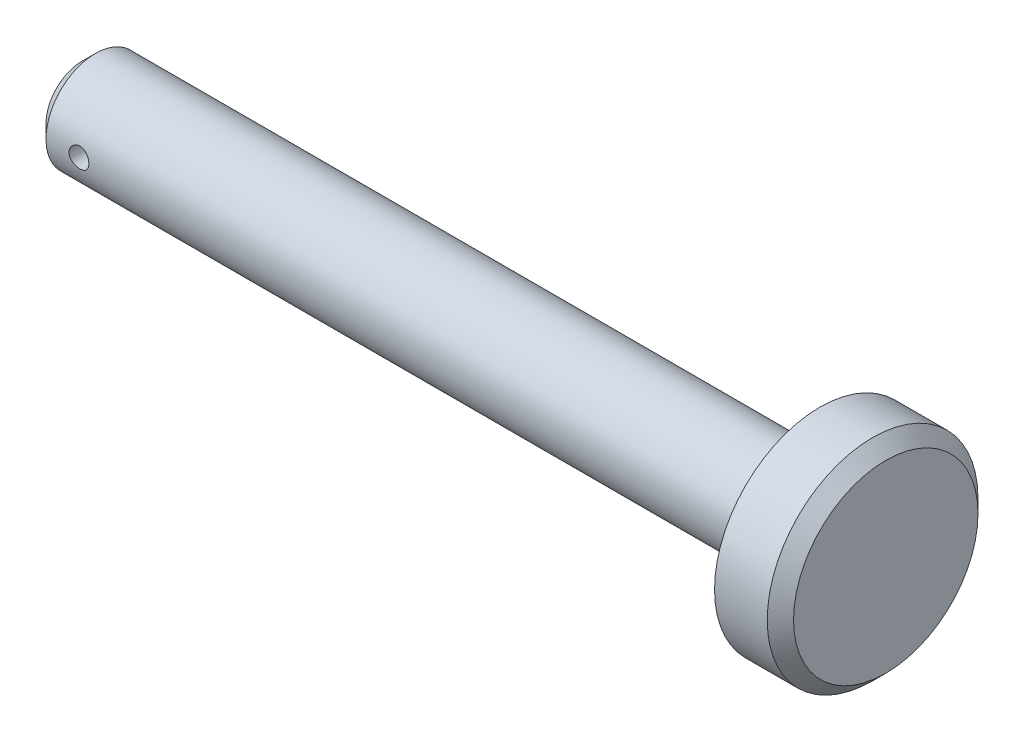
ISO-10303-21;
HEADER;
FILE_DESCRIPTION(('STEP AP214'),'2;1');
FILE_NAME('part.step','',(''),(''),'','','');
FILE_SCHEMA(('AUTOMOTIVE_DESIGN { 1 0 10303 214 1 1 1 1 }'));
ENDSEC;
DATA;
#1=APPLICATION_CONTEXT('core data for automotive mechanical design processes');
#2=APPLICATION_PROTOCOL_DEFINITION('international standard','automotive_design',2000,#1);
#3=PRODUCT_CONTEXT('',#1,'mechanical');
#4=PRODUCT('Part','Part','',(#3));
#5=PRODUCT_RELATED_PRODUCT_CATEGORY('part','',(#4));
#6=PRODUCT_DEFINITION_FORMATION('','',#4);
#7=PRODUCT_DEFINITION_CONTEXT('part definition',#1,'design');
#8=PRODUCT_DEFINITION('design','',#6,#7);
#9=PRODUCT_DEFINITION_SHAPE('','',#8);
#10=(LENGTH_UNIT() NAMED_UNIT(*) SI_UNIT(.MILLI.,.METRE.));
#11=(NAMED_UNIT(*) PLANE_ANGLE_UNIT() SI_UNIT($,.RADIAN.));
#12=(NAMED_UNIT(*) SI_UNIT($,.STERADIAN.) SOLID_ANGLE_UNIT());
#13=UNCERTAINTY_MEASURE_WITH_UNIT(LENGTH_MEASURE(1.E-05),#10,'distance_accuracy_value','');
#14=(GEOMETRIC_REPRESENTATION_CONTEXT(3) GLOBAL_UNCERTAINTY_ASSIGNED_CONTEXT((#13)) GLOBAL_UNIT_ASSIGNED_CONTEXT((#10,
#11,#12)) REPRESENTATION_CONTEXT('',''));
#15=CARTESIAN_POINT('',(0.,0.,0.));
#16=DIRECTION('',(0.,0.,1.));
#17=DIRECTION('',(1.,0.,0.));
#18=AXIS2_PLACEMENT_3D('',#15,#16,#17);
#19=CARTESIAN_POINT('',(0.,0.,0.));
#20=DIRECTION('',(1.,0.,0.));
#21=DIRECTION('',(0.,1.,0.));
#22=AXIS2_PLACEMENT_3D('',#19,#20,#21);
#23=PLANE('',#22);
#24=CARTESIAN_POINT('',(0.,0.,0.));
#25=DIRECTION('',(1.,0.,0.));
#26=DIRECTION('',(0.,1.,0.));
#27=AXIS2_PLACEMENT_3D('',#24,#25,#26);
#28=CIRCLE('',#27,5.49999999999999);
#29=CARTESIAN_POINT('',(0.,5.49999999999999,0.));
#30=VERTEX_POINT('',#29);
#31=EDGE_CURVE('E51',#30,#30,#28,.F.);
#32=ORIENTED_EDGE('',*,*,#31,.T.);
#33=EDGE_LOOP('',(#32));
#34=FACE_BOUND('',#33,.T.);
#35=ADVANCED_FACE('F39',(#34),#23,.F.);
#36=CARTESIAN_POINT('',(122.,0.,0.));
#37=DIRECTION('',(1.,0.,0.));
#38=DIRECTION('',(0.,1.,0.));
#39=AXIS2_PLACEMENT_3D('',#36,#37,#38);
#40=CYLINDRICAL_SURFACE('',#39,7.5);
#41=CARTESIAN_POINT('',(1.99999999999999,0.,0.));
#42=DIRECTION('',(1.,0.,0.));
#43=DIRECTION('',(0.,1.,0.));
#44=AXIS2_PLACEMENT_3D('',#41,#42,#43);
#45=CIRCLE('',#44,7.5);
#46=CARTESIAN_POINT('',(1.99999999999999,7.5,0.));
#47=VERTEX_POINT('',#46);
#48=EDGE_CURVE('E54',#47,#47,#45,.T.);
#49=ORIENTED_EDGE('',*,*,#48,.T.);
#50=EDGE_LOOP('',(#49));
#51=FACE_BOUND('',#50,.T.);
#52=CARTESIAN_POINT('',(8.50000000000001,0.,-7.5));
#53=CARTESIAN_POINT('',(8.49999693325249,0.0833653601889498,-7.49999846371307));
#54=CARTESIAN_POINT('',(8.49302673554854,0.166769490302284,-7.49859577767347));
#55=CARTESIAN_POINT('',(8.46535224982714,0.331220261533529,-7.49313548434847));
#56=CARTESIAN_POINT('',(8.44463705079774,0.412264976312034,-7.48907576790279));
#57=CARTESIAN_POINT('',(8.39013808956882,0.56959545789497,-7.4787547391743));
#58=CARTESIAN_POINT('',(8.35636684473297,0.645885701899702,-7.47249553615077));
#59=CARTESIAN_POINT('',(8.27675162873306,0.791711983296339,-7.45845597052972));
#60=CARTESIAN_POINT('',(8.2309083765892,0.861248422613719,-7.4506756985356));
#61=CARTESIAN_POINT('',(8.12779225856286,0.992540215972299,-7.43433247994955));
#62=CARTESIAN_POINT('',(8.0703874669132,1.05419092673779,-7.42576118256521));
#63=CARTESIAN_POINT('',(7.94606137541245,1.16705513491204,-7.40886270678883));
#64=CARTESIAN_POINT('',(7.87913933299733,1.21826781715564,-7.40053554750636));
#65=CARTESIAN_POINT('',(7.73692571048219,1.30924763002143,-7.38498662718923));
#66=CARTESIAN_POINT('',(7.66156353430547,1.3489064082988,-7.37777561047419));
#67=CARTESIAN_POINT('',(7.50507727149389,1.41495849987046,-7.36539402087627));
#68=CARTESIAN_POINT('',(7.42395375498049,1.44135312365586,-7.36022324642943));
#69=CARTESIAN_POINT('',(7.25937345413813,1.47978794982724,-7.35259207878307));
#70=CARTESIAN_POINT('',(7.17596118378667,1.49201174693817,-7.35009705160782));
#71=CARTESIAN_POINT('',(7.00823526795349,1.50232819158918,-7.34799562590941));
#72=CARTESIAN_POINT('',(6.92392171551979,1.50042228407025,-7.34838893201761));
#73=CARTESIAN_POINT('',(6.7581298179685,1.48268185965273,-7.35198826722277));
#74=CARTESIAN_POINT('',(6.67662789155904,1.46705781036586,-7.35515179288145));
#75=CARTESIAN_POINT('',(6.5174258850055,1.42265682693458,-7.36386819240002));
#76=CARTESIAN_POINT('',(6.43972598662149,1.39387926465102,-7.36942118036668));
#77=CARTESIAN_POINT('',(6.28972710744461,1.32378717551208,-7.38233427750612));
#78=CARTESIAN_POINT('',(6.21746818064625,1.28238922684817,-7.38970634720557));
#79=CARTESIAN_POINT('',(6.08084372504079,1.18829036185902,-7.40541928159593));
#80=CARTESIAN_POINT('',(6.01647910472327,1.13558814653524,-7.41376025757549));
#81=CARTESIAN_POINT('',(5.8962558963146,1.01924990184088,-7.43065531862193));
#82=CARTESIAN_POINT('',(5.84057114821131,0.955434241818668,-7.43921053816357));
#83=CARTESIAN_POINT('',(5.74066923054817,0.819277536093015,-7.45543273071613));
#84=CARTESIAN_POINT('',(5.69645220805964,0.746936381069084,-7.46309969233461));
#85=CARTESIAN_POINT('',(5.62070873616104,0.595589080318381,-7.47670035241331));
#86=CARTESIAN_POINT('',(5.5892021595332,0.51657272937795,-7.48263133272408));
#87=CARTESIAN_POINT('',(5.53995928894216,0.354223464672997,-7.49207113481788));
#88=CARTESIAN_POINT('',(5.52222132688956,0.270891075108674,-7.49558025000797));
#89=CARTESIAN_POINT('',(5.50126531930859,0.103769108440726,-7.49974007800302));
#90=CARTESIAN_POINT('',(5.4978093706896,0.0200104924883642,-7.50043761978705));
#91=CARTESIAN_POINT('',(5.50487478841328,-0.146887401289071,-7.49902577895154));
#92=CARTESIAN_POINT('',(5.5153953690289,-0.23002671366569,-7.49691655412169));
#93=CARTESIAN_POINT('',(5.54991756031594,-0.392558489919812,-7.49015748012027));
#94=CARTESIAN_POINT('',(5.57379710274686,-0.471977922509855,-7.4855306460631));
#95=CARTESIAN_POINT('',(5.63422597398372,-0.625685441249501,-7.47425328091549));
#96=CARTESIAN_POINT('',(5.67077625201525,-0.69997314245631,-7.4676025982134));
#97=CARTESIAN_POINT('',(5.75602373597697,-0.842311760529327,-7.45289867299942));
#98=CARTESIAN_POINT('',(5.80486417155842,-0.910275190128282,-7.44482925655578));
#99=CARTESIAN_POINT('',(5.91311378681093,-1.03712702867881,-7.42822102244824));
#100=CARTESIAN_POINT('',(5.97252409959981,-1.09601446339614,-7.41968215452582));
#101=CARTESIAN_POINT('',(6.10131002783669,-1.20396088616126,-7.40293955335448));
#102=CARTESIAN_POINT('',(6.17082361633201,-1.25285655367298,-7.39474290349956));
#103=CARTESIAN_POINT('',(6.31721704203502,-1.33827813007681,-7.37976287694292));
#104=CARTESIAN_POINT('',(6.39409658436033,-1.37480453388435,-7.37297944370014));
#105=CARTESIAN_POINT('',(6.55265236922433,-1.43422776237294,-7.36165110876574));
#106=CARTESIAN_POINT('',(6.63430126181549,-1.45719524968658,-7.3570946230828));
#107=CARTESIAN_POINT('',(6.80040018023637,-1.48906297744079,-7.35071155188038));
#108=CARTESIAN_POINT('',(6.88484983931403,-1.49796505233767,-7.34888461036667));
#109=CARTESIAN_POINT('',(7.05251329681648,-1.5013813663012,-7.34818724447069));
#110=CARTESIAN_POINT('',(7.13572172339052,-1.49615368210634,-7.34926378783951));
#111=CARTESIAN_POINT('',(7.30004747485755,-1.47202845615009,-7.35413360226921));
#112=CARTESIAN_POINT('',(7.38116481654221,-1.45313102419395,-7.35792685150754));
#113=CARTESIAN_POINT('',(7.53884156686082,-1.40231785274843,-7.36777896328738));
#114=CARTESIAN_POINT('',(7.61541154075363,-1.37043376007602,-7.37383231528246));
#115=CARTESIAN_POINT('',(7.76215558110167,-1.29458196690241,-7.38752572461255));
#116=CARTESIAN_POINT('',(7.83232911058771,-1.25061325316232,-7.39516591498341));
#117=CARTESIAN_POINT('',(7.96557335822548,-1.15095887217962,-7.41133440784838));
#118=CARTESIAN_POINT('',(8.0285031479014,-1.09508683085277,-7.41987559364549));
#119=CARTESIAN_POINT('',(8.14417930829377,-0.97359655351971,-7.43679122807932));
#120=CARTESIAN_POINT('',(8.19692333547592,-0.907976080730002,-7.44516563794777));
#121=CARTESIAN_POINT('',(8.29125196591968,-0.76802644363237,-7.46090748581957));
#122=CARTESIAN_POINT('',(8.33271400492005,-0.693613326644752,-7.46826346828869));
#123=CARTESIAN_POINT('',(8.4024791838949,-0.538749541411099,-7.481026876275));
#124=CARTESIAN_POINT('',(8.43079418429875,-0.45830439129469,-7.48643605707924));
#125=CARTESIAN_POINT('',(8.46797792206708,-0.314732233385669,-7.49364558893056));
#126=CARTESIAN_POINT('',(8.47996479056164,-0.252422496020677,-7.49601454737678));
#127=CARTESIAN_POINT('',(8.49597686853755,-0.1267492878151,-7.49919231209839));
#128=CARTESIAN_POINT('',(8.50000233176466,-0.0633858506229285,-7.50000116809733));
#129=CARTESIAN_POINT('',(8.50000000000001,0.,-7.5));
#130=B_SPLINE_CURVE_WITH_KNOTS('',3,(#52,#53,#54,#55,#56,#57,#58,#59,#60,#61,#62,#63,#64,#65,
#66,#67,#68,#69,#70,#71,#72,#73,#74,#75,#76,#77,#78,#79,#80,#81,#82,#83,#84,#85,#86,#87,#88,#89,
#90,#91,#92,#93,#94,#95,#96,#97,#98,#99,#100,#101,#102,#103,#104,#105,#106,#107,#108,#109,#110,
#111,#112,#113,#114,#115,#116,#117,#118,#119,#120,#121,#122,#123,#124,#125,#126,#127,#128,#129),
.UNSPECIFIED.,.T.,.F.,(4,2,2,2,2,2,2,2,2,2,2,2,2,2,2,2,2,2,2,2,2,2,2,2,2,2,2,2,2,2,2,2,2,2,2,2,
2,2,4),(0.,0.249864195991888,0.499926976036985,0.749750602875513,0.999559353346296,
1.25239900516828,1.50525839512105,1.76041792508884,2.01555224047796,2.26734277655381,
2.51910756421838,2.76707590509418,3.01505608880595,3.26471235305389,3.51439732124506,
3.76857378737026,4.0227535130973,4.27732912281036,4.53187388547054,4.78216103514398,
5.03243411486801,5.28045680926085,5.52849808824034,5.77957599050038,6.03068082518895,
6.28560942868839,6.540527830852,6.79410571549085,7.04765052495622,7.29659583851552,
7.54553915238913,7.79387941879665,8.042240513728,8.29482114358715,8.54745981799396,
8.80274245013456,9.05779433276278,9.24778162934841,9.43776287056494),.UNSPECIFIED.);
#131=CARTESIAN_POINT('',(8.50000000000001,0.,-7.5));
#132=VERTEX_POINT('',#131);
#133=EDGE_CURVE('E61',#132,#132,#130,.T.);
#134=ORIENTED_EDGE('',*,*,#133,.T.);
#135=EDGE_LOOP('',(#134));
#136=FACE_BOUND('',#135,.T.);
#137=CARTESIAN_POINT('',(8.50000000000001,0.,7.5));
#138=CARTESIAN_POINT('',(8.49999693325249,-0.0833653601889498,7.49999846371307));
#139=CARTESIAN_POINT('',(8.49302673554854,-0.166769490302283,7.49859577767347));
#140=CARTESIAN_POINT('',(8.46535224982714,-0.331220261533529,7.49313548434847));
#141=CARTESIAN_POINT('',(8.44463705079774,-0.412264976312034,7.48907576790279));
#142=CARTESIAN_POINT('',(8.39013808956882,-0.56959545789497,7.4787547391743));
#143=CARTESIAN_POINT('',(8.35636684473297,-0.645885701899702,7.47249553615077));
#144=CARTESIAN_POINT('',(8.27675162873306,-0.791711983296339,7.45845597052972));
#145=CARTESIAN_POINT('',(8.2309083765892,-0.861248422613719,7.4506756985356));
#146=CARTESIAN_POINT('',(8.12779225856286,-0.992540215972299,7.43433247994955));
#147=CARTESIAN_POINT('',(8.0703874669132,-1.05419092673779,7.42576118256521));
#148=CARTESIAN_POINT('',(7.94606137541245,-1.16705513491204,7.40886270678883));
#149=CARTESIAN_POINT('',(7.87913933299733,-1.21826781715564,7.40053554750636));
#150=CARTESIAN_POINT('',(7.73692571048219,-1.30924763002143,7.38498662718923));
#151=CARTESIAN_POINT('',(7.66156353430547,-1.3489064082988,7.37777561047419));
#152=CARTESIAN_POINT('',(7.50507727149389,-1.41495849987046,7.36539402087627));
#153=CARTESIAN_POINT('',(7.42395375498049,-1.44135312365586,7.36022324642943));
#154=CARTESIAN_POINT('',(7.25937345413813,-1.47978794982724,7.35259207878307));
#155=CARTESIAN_POINT('',(7.17596118378667,-1.49201174693817,7.35009705160782));
#156=CARTESIAN_POINT('',(7.00823526795349,-1.50232819158918,7.34799562590941));
#157=CARTESIAN_POINT('',(6.92392171551979,-1.50042228407025,7.34838893201761));
#158=CARTESIAN_POINT('',(6.7581298179685,-1.48268185965273,7.35198826722277));
#159=CARTESIAN_POINT('',(6.67662789155904,-1.46705781036586,7.35515179288145));
#160=CARTESIAN_POINT('',(6.5174258850055,-1.42265682693458,7.36386819240002));
#161=CARTESIAN_POINT('',(6.43972598662149,-1.39387926465102,7.36942118036668));
#162=CARTESIAN_POINT('',(6.28972710744461,-1.32378717551208,7.38233427750612));
#163=CARTESIAN_POINT('',(6.21746818064625,-1.28238922684817,7.38970634720557));
#164=CARTESIAN_POINT('',(6.08084372504079,-1.18829036185902,7.40541928159593));
#165=CARTESIAN_POINT('',(6.01647910472327,-1.13558814653524,7.41376025757549));
#166=CARTESIAN_POINT('',(5.8962558963146,-1.01924990184088,7.43065531862193));
#167=CARTESIAN_POINT('',(5.84057114821131,-0.955434241818668,7.43921053816357));
#168=CARTESIAN_POINT('',(5.74066923054817,-0.819277536093015,7.45543273071613));
#169=CARTESIAN_POINT('',(5.69645220805964,-0.746936381069084,7.4630996923346));
#170=CARTESIAN_POINT('',(5.62070873616104,-0.595589080318381,7.47670035241331));
#171=CARTESIAN_POINT('',(5.5892021595332,-0.51657272937795,7.48263133272408));
#172=CARTESIAN_POINT('',(5.53995928894216,-0.354223464672997,7.49207113481788));
#173=CARTESIAN_POINT('',(5.52222132688956,-0.270891075108674,7.49558025000797));
#174=CARTESIAN_POINT('',(5.50126531930859,-0.103769108440725,7.49974007800302));
#175=CARTESIAN_POINT('',(5.4978093706896,-0.0200104924883638,7.50043761978705));
#176=CARTESIAN_POINT('',(5.50487478841328,0.146887401289072,7.49902577895154));
#177=CARTESIAN_POINT('',(5.5153953690289,0.23002671366569,7.49691655412169));
#178=CARTESIAN_POINT('',(5.54991756031594,0.392558489919812,7.49015748012027));
#179=CARTESIAN_POINT('',(5.57379710274686,0.471977922509855,7.4855306460631));
#180=CARTESIAN_POINT('',(5.63422597398372,0.625685441249501,7.47425328091549));
#181=CARTESIAN_POINT('',(5.67077625201525,0.69997314245631,7.4676025982134));
#182=CARTESIAN_POINT('',(5.75602373597698,0.842311760529327,7.45289867299942));
#183=CARTESIAN_POINT('',(5.80486417155842,0.910275190128282,7.44482925655578));
#184=CARTESIAN_POINT('',(5.91311378681093,1.03712702867881,7.42822102244824));
#185=CARTESIAN_POINT('',(5.97252409959981,1.09601446339614,7.41968215452582));
#186=CARTESIAN_POINT('',(6.10131002783669,1.20396088616126,7.40293955335448));
#187=CARTESIAN_POINT('',(6.17082361633201,1.25285655367298,7.39474290349956));
#188=CARTESIAN_POINT('',(6.31721704203503,1.33827813007681,7.37976287694292));
#189=CARTESIAN_POINT('',(6.39409658436034,1.37480453388436,7.37297944370014));
#190=CARTESIAN_POINT('',(6.55265236922433,1.43422776237294,7.36165110876574));
#191=CARTESIAN_POINT('',(6.63430126181549,1.45719524968658,7.3570946230828));
#192=CARTESIAN_POINT('',(6.80040018023637,1.48906297744079,7.35071155188038));
#193=CARTESIAN_POINT('',(6.88484983931403,1.49796505233767,7.34888461036667));
#194=CARTESIAN_POINT('',(7.05251329681648,1.5013813663012,7.34818724447069));
#195=CARTESIAN_POINT('',(7.13572172339052,1.49615368210634,7.34926378783952));
#196=CARTESIAN_POINT('',(7.30004747485755,1.47202845615009,7.35413360226921));
#197=CARTESIAN_POINT('',(7.38116481654221,1.45313102419395,7.35792685150754));
#198=CARTESIAN_POINT('',(7.53884156686082,1.40231785274843,7.36777896328738));
#199=CARTESIAN_POINT('',(7.61541154075363,1.37043376007602,7.37383231528246));
#200=CARTESIAN_POINT('',(7.76215558110167,1.29458196690241,7.38752572461255));
#201=CARTESIAN_POINT('',(7.83232911058771,1.25061325316232,7.39516591498341));
#202=CARTESIAN_POINT('',(7.96557335822548,1.15095887217962,7.41133440784838));
#203=CARTESIAN_POINT('',(8.0285031479014,1.09508683085277,7.41987559364549));
#204=CARTESIAN_POINT('',(8.14417930829377,0.97359655351971,7.43679122807932));
#205=CARTESIAN_POINT('',(8.19692333547591,0.907976080730002,7.44516563794777));
#206=CARTESIAN_POINT('',(8.29125196591968,0.76802644363237,7.46090748581957));
#207=CARTESIAN_POINT('',(8.33271400492005,0.693613326644752,7.46826346828869));
#208=CARTESIAN_POINT('',(8.4024791838949,0.538749541411099,7.481026876275));
#209=CARTESIAN_POINT('',(8.43079418429874,0.45830439129469,7.48643605707924));
#210=CARTESIAN_POINT('',(8.46797792206708,0.314732233385669,7.49364558893056));
#211=CARTESIAN_POINT('',(8.47996479056164,0.252422496020677,7.49601454737678));
#212=CARTESIAN_POINT('',(8.49597686853755,0.1267492878151,7.49919231209839));
#213=CARTESIAN_POINT('',(8.50000233176466,0.0633858506229283,7.50000116809733));
#214=CARTESIAN_POINT('',(8.50000000000001,0.,7.5));
#215=B_SPLINE_CURVE_WITH_KNOTS('',3,(#137,#138,#139,#140,#141,#142,#143,#144,#145,#146,#147,
#148,#149,#150,#151,#152,#153,#154,#155,#156,#157,#158,#159,#160,#161,#162,#163,#164,#165,#166,
#167,#168,#169,#170,#171,#172,#173,#174,#175,#176,#177,#178,#179,#180,#181,#182,#183,#184,#185,
#186,#187,#188,#189,#190,#191,#192,#193,#194,#195,#196,#197,#198,#199,#200,#201,#202,#203,#204,
#205,#206,#207,#208,#209,#210,#211,#212,#213,#214),.UNSPECIFIED.,.T.,.F.,(4,2,2,2,2,2,2,2,2,2,2,
2,2,2,2,2,2,2,2,2,2,2,2,2,2,2,2,2,2,2,2,2,2,2,2,2,2,2,4),(0.,0.249864195991888,
0.499926976036985,0.749750602875513,0.999559353346296,1.25239900516828,1.50525839512105,
1.76041792508884,2.01555224047796,2.26734277655381,2.51910756421838,2.76707590509418,
3.01505608880595,3.26471235305389,3.51439732124506,3.76857378737026,4.0227535130973,
4.27732912281036,4.53187388547054,4.78216103514398,5.03243411486801,5.28045680926085,
5.52849808824034,5.77957599050038,6.03068082518895,6.28560942868839,6.540527830852,
6.79410571549085,7.04765052495622,7.29659583851552,7.54553915238913,7.79387941879665,
8.042240513728,8.29482114358715,8.54745981799396,8.80274245013456,9.05779433276278,
9.24778162934841,9.43776287056495),.UNSPECIFIED.);
#216=CARTESIAN_POINT('',(8.50000000000001,0.,7.5));
#217=VERTEX_POINT('',#216);
#218=EDGE_CURVE('E69',#217,#217,#215,.T.);
#219=ORIENTED_EDGE('',*,*,#218,.T.);
#220=EDGE_LOOP('',(#219));
#221=FACE_BOUND('',#220,.T.);
#222=CARTESIAN_POINT('',(112.,0.,0.));
#223=DIRECTION('',(1.,0.,0.));
#224=DIRECTION('',(0.,1.,0.));
#225=AXIS2_PLACEMENT_3D('',#222,#223,#224);
#226=CIRCLE('',#225,7.5);
#227=CARTESIAN_POINT('',(112.,7.50000000000001,0.));
#228=VERTEX_POINT('',#227);
#229=EDGE_CURVE('E58',#228,#228,#226,.T.);
#230=ORIENTED_EDGE('',*,*,#229,.F.);
#231=EDGE_LOOP('',(#230));
#232=FACE_BOUND('',#231,.T.);
#233=ADVANCED_FACE('F73',(#51,#136,#221,#232),#40,.T.);
#234=CARTESIAN_POINT('',(112.,-7.5,0.));
#235=DIRECTION('',(1.,0.,0.));
#236=DIRECTION('',(0.,1.,0.));
#237=AXIS2_PLACEMENT_3D('',#234,#235,#236);
#238=PLANE('',#237);
#239=CARTESIAN_POINT('',(112.,0.,0.));
#240=DIRECTION('',(1.,0.,0.));
#241=DIRECTION('',(0.,1.,0.));
#242=AXIS2_PLACEMENT_3D('',#239,#240,#241);
#243=CIRCLE('',#242,16.);
#244=CARTESIAN_POINT('',(112.,16.,0.));
#245=VERTEX_POINT('',#244);
#246=EDGE_CURVE('E67',#245,#245,#243,.T.);
#247=ORIENTED_EDGE('',*,*,#246,.F.);
#248=EDGE_LOOP('',(#247));
#249=FACE_BOUND('',#248,.T.);
#250=ORIENTED_EDGE('',*,*,#229,.T.);
#251=EDGE_LOOP('',(#250));
#252=FACE_BOUND('',#251,.T.);
#253=ADVANCED_FACE('F93',(#249,#252),#238,.F.);
#254=CARTESIAN_POINT('',(122.,0.,0.));
#255=DIRECTION('',(1.,0.,0.));
#256=DIRECTION('',(0.,1.,0.));
#257=AXIS2_PLACEMENT_3D('',#254,#255,#256);
#258=CYLINDRICAL_SURFACE('',#257,16.);
#259=CARTESIAN_POINT('',(120.,0.,0.));
#260=DIRECTION('',(-1.,0.,0.));
#261=DIRECTION('',(0.,-1.,0.));
#262=AXIS2_PLACEMENT_3D('',#259,#260,#261);
#263=CIRCLE('',#262,16.);
#264=CARTESIAN_POINT('',(120.,-16.,0.));
#265=VERTEX_POINT('',#264);
#266=EDGE_CURVE('E10',#265,#265,#263,.T.);
#267=ORIENTED_EDGE('',*,*,#266,.T.);
#268=EDGE_LOOP('',(#267));
#269=FACE_BOUND('',#268,.T.);
#270=ORIENTED_EDGE('',*,*,#246,.T.);
#271=EDGE_LOOP('',(#270));
#272=FACE_BOUND('',#271,.T.);
#273=ADVANCED_FACE('F90',(#269,#272),#258,.T.);
#274=CARTESIAN_POINT('',(122.,-16.,0.));
#275=DIRECTION('',(-1.,0.,0.));
#276=DIRECTION('',(0.,-1.,0.));
#277=AXIS2_PLACEMENT_3D('',#274,#275,#276);
#278=PLANE('',#277);
#279=CARTESIAN_POINT('',(122.,0.,0.));
#280=DIRECTION('',(-1.,0.,0.));
#281=DIRECTION('',(0.,-1.,0.));
#282=AXIS2_PLACEMENT_3D('',#279,#280,#281);
#283=CIRCLE('',#282,14.);
#284=CARTESIAN_POINT('',(122.,-14.,0.));
#285=VERTEX_POINT('',#284);
#286=EDGE_CURVE('E50',#285,#285,#283,.F.);
#287=ORIENTED_EDGE('',*,*,#286,.T.);
#288=EDGE_LOOP('',(#287));
#289=FACE_BOUND('',#288,.T.);
#290=ADVANCED_FACE('F82',(#289),#278,.F.);
#291=CARTESIAN_POINT('',(7.00000000000001,0.,-16.));
#292=DIRECTION('',(0.,0.,1.));
#293=DIRECTION('',(1.,0.,0.));
#294=AXIS2_PLACEMENT_3D('',#291,#292,#293);
#295=CYLINDRICAL_SURFACE('',#294,1.5);
#296=ORIENTED_EDGE('',*,*,#218,.F.);
#297=EDGE_LOOP('',(#296));
#298=FACE_BOUND('',#297,.T.);
#299=ORIENTED_EDGE('',*,*,#133,.F.);
#300=EDGE_LOOP('',(#299));
#301=FACE_BOUND('',#300,.T.);
#302=ADVANCED_FACE('F78',(#298,#301),#295,.F.);
#303=CARTESIAN_POINT('',(1.99999999999999,0.,0.));
#304=DIRECTION('',(1.,0.,0.));
#305=DIRECTION('',(0.,1.,0.));
#306=AXIS2_PLACEMENT_3D('',#303,#304,#305);
#307=CONICAL_SURFACE('',#306,7.5,0.785398163397454);
#308=ORIENTED_EDGE('',*,*,#31,.F.);
#309=EDGE_LOOP('',(#308));
#310=FACE_BOUND('',#309,.T.);
#311=ORIENTED_EDGE('',*,*,#48,.F.);
#312=EDGE_LOOP('',(#311));
#313=FACE_BOUND('',#312,.T.);
#314=ADVANCED_FACE('F83',(#310,#313),#307,.T.);
#315=CARTESIAN_POINT('',(122.,0.,0.));
#316=DIRECTION('',(-1.,0.,0.));
#317=DIRECTION('',(0.,-1.,0.));
#318=AXIS2_PLACEMENT_3D('',#315,#316,#317);
#319=CONICAL_SURFACE('',#318,14.,0.785398163397445);
#320=ORIENTED_EDGE('',*,*,#266,.F.);
#321=EDGE_LOOP('',(#320));
#322=FACE_BOUND('',#321,.T.);
#323=ORIENTED_EDGE('',*,*,#286,.F.);
#324=EDGE_LOOP('',(#323));
#325=FACE_BOUND('',#324,.T.);
#326=ADVANCED_FACE('F45',(#322,#325),#319,.T.);
#327=CLOSED_SHELL('',(#35,#233,#253,#273,#290,#302,#314,#326));
#328=MANIFOLD_SOLID_BREP('B2',#327);
#329=ADVANCED_BREP_SHAPE_REPRESENTATION('',(#18,#328),#14);
#330=SHAPE_DEFINITION_REPRESENTATION(#9,#329);
ENDSEC;
END-ISO-10303-21;
